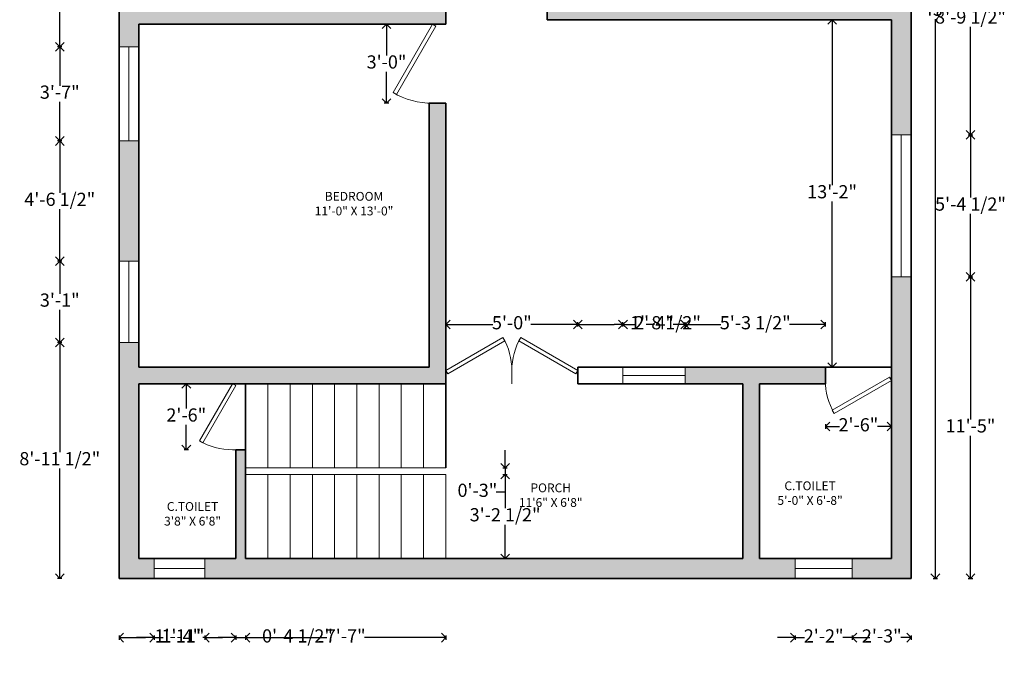
# Model space of a CAD drawing. Units: inches. Extents: x 2542 to 2989, y 529 to 1112.
# Tile 1 of 2: x 2542 to 2989, y 529 to 819. Entities that reach past the tile are written whole.
import ezdxf

# ---------------------------------------------------------------- set-up
doc = ezdxf.new("R2010")
doc.units = ezdxf.units.IN
for name, color, linetype, lineweight in [('A-ANNO-DIMS', 2, 'Continuous', 18), ('A-AREA-IDEN', 7, 'Continuous', 18), ('A-DOOR', 3, 'Continuous', 18), ('A-FLOR-STRS', 7, 'Continuous', 18), ('A-GLAZ', 4, 'Continuous', 18), ('A-WALL', 7, 'Continuous', 35)]:
    doc.layers.add(name, color=color, linetype=linetype, lineweight=lineweight)
doc.layers.add('A-WALL-PATT', color=30, linetype='Continuous', lineweight=13, true_color=0xf26722)
doc.styles.get("Standard").update_dxf_attribs({"font": 'arial.ttf'})
doc.dimstyles.new('ISO-25', dxfattribs={"dimtxt": 6, "dimasz": 4, "dimexe": 1, "dimexo": 1, "dimtad": 0, "dimtih": 1, "dimtoh": 1, "dimlunit": 3, "dimtxsty": 'Standard', "dimblk": 'OPEN90', "dimcen": 2.5, "dimadec": 0, "dimazin": 0, "dimtfac": 1, "dimtmove": 0, "dimatfit": 3, "dimfxl": 1, "dimfxlon": 1, "dimarcsym": 0})

# ---------------------------------------------------------------- blocks, each defined once
blk = doc.blocks.new('*U8')
for p, q in [((-30, 0), (-30, -6)), ((0, 0), (0, -6))]:
    blk.add_line(p, q)
blk.add_lwpolyline([(0, 0), (-25.98, 15), (-26.86, 13.48), (-0.88, -1.52)], close=True)
blk.add_arc((0, 0), 30, 150, 180)
blk = doc.blocks.new('*U9')
for p, q in [((0, 0), (0, -6)), ((30, 0), (30, -6))]:
    blk.add_line(p, q)
blk.add_lwpolyline([(0, 0), (25.98, 15), (26.86, 13.48), (0.87, -1.52)], close=True)
blk.add_arc((0, 0), 30, 0, 30)
blk = doc.blocks.new('*U6')
for p, q in [((-30, 0), (-30, 6)), ((0, 0), (0, 6))]:
    blk.add_line(p, q)
blk.add_lwpolyline([(0, 0), (-25.98, -15), (-26.86, -13.48), (-0.88, 1.52)], close=True)
blk.add_arc((0, 0), 30, 180, 210)
blk = doc.blocks.new('*U7')
for p, q in [((0, 0), (0, 6)), ((30, 0), (30, 6))]:
    blk.add_line(p, q)
blk.add_lwpolyline([(0, 0), (25.98, -15), (26.86, -13.48), (0.87, 1.52)], close=True)
blk.add_arc((0, 0), 30, 330, 0)
blk = doc.blocks.new('*U4')
for p, q in [((0, 0), (0, -6)), ((-36, 0), (-36, -6))]:
    blk.add_line(p, q)
blk.add_lwpolyline([(0, 0), (-31.18, 18), (-32.05, 16.48), (-0.88, -1.52)], close=True)
blk.add_arc((0, 0), 36, 150, 180)
blk = doc.blocks.new('_Open90')
at = {"color": 0, "linetype": 'ByBlock', "lineweight": -2}
for p, q in [((0, 0), (-1, 0)), ((-0.5, 0.5), (0, 0)), ((0, 0), (-0.5, -0.5))]:
    blk.add_line(p, q, dxfattribs=at)
blk = doc.blocks.new('*D13')
at = {"layer": 'A-ANNO-DIMS', "color": 0, "lineweight": -2, "transparency": 16777216}
for p, q in [((2957.03, 1081), (2959.03, 1081)), ((2958.03, 1077), (2958.03, 826.69)), ((2958.03, 569), (2958.03, 819.31)), ((2957.03, 565), (2959.03, 565))]:
    blk.add_line(p, q, dxfattribs=at)
at = {"layer": 'Defpoints', "color": 0, "transparency": 16777216}
for p in [(2947.06, 1081), (2947.06, 565), (2958.03, 565)]:
    blk.add_point(p, dxfattribs=at)
at = {"layer": 'A-ANNO-DIMS', "color": 0, "lineweight": -2, "transparency": 16777216, "xscale": 4, "yscale": 4, "zscale": 4}
for p, rotation in [((2958.03, 1081), 90), ((2958.03, 565), 270)]:
    blk.add_blockref('_Open90', p, dxfattribs=dict(at, rotation=rotation))
at = {"layer": 'A-ANNO-DIMS', "color": 0, "transparency": 16777216, "insert": (2958.03, 823), "char_height": 6, "attachment_point": 5}
blk.add_mtext("43'", dxfattribs=at)
blk = doc.blocks.new('*D14')
at = {"layer": 'A-ANNO-DIMS', "color": 0, "lineweight": -2, "transparency": 16777216}
for p, q in [((2561.11, 672.25), (2559.11, 672.25)), ((2560.11, 668.25), (2560.11, 622.35)), ((2560.11, 569), (2560.11, 614.9)), ((2561.11, 565), (2559.11, 565))]:
    blk.add_line(p, q, dxfattribs=at)
at = {"layer": 'Defpoints', "color": 0, "transparency": 16777216}
for p in [(2560.11, 672.25), (2587.06, 672.25), (2587.06, 565)]:
    blk.add_point(p, dxfattribs=at)
at = {"layer": 'A-ANNO-DIMS', "color": 0, "lineweight": -2, "transparency": 16777216, "xscale": 4, "yscale": 4, "zscale": 4}
for p, rotation in [((2560.11, 672.25), 90), ((2560.11, 565), 270)]:
    blk.add_blockref('_Open90', p, dxfattribs=dict(at, rotation=rotation))
at = {"layer": 'A-ANNO-DIMS', "color": 0, "transparency": 16777216, "insert": (2560.11, 618.63), "char_height": 6, "attachment_point": 5}
blk.add_mtext('8\'-11 1/2"', dxfattribs=at)
blk = doc.blocks.new('*D15')
at = {"layer": 'A-ANNO-DIMS', "color": 0, "lineweight": -2, "transparency": 16777216}
for p, q in [((2561.11, 709.22), (2559.11, 709.22)), ((2560.11, 705.22), (2560.11, 694.43)), ((2560.11, 676.25), (2560.11, 687.05)), ((2561.11, 672.25), (2559.11, 672.25))]:
    blk.add_line(p, q, dxfattribs=at)
at = {"layer": 'Defpoints', "color": 0, "transparency": 16777216}
for p in [(2560.11, 709.22), (2587.06, 709.22), (2587.06, 672.25)]:
    blk.add_point(p, dxfattribs=at)
at = {"layer": 'A-ANNO-DIMS', "color": 0, "lineweight": -2, "transparency": 16777216, "xscale": 4, "yscale": 4, "zscale": 4}
for p, rotation in [((2560.11, 709.22), 90), ((2560.11, 672.25), 270)]:
    blk.add_blockref('_Open90', p, dxfattribs=dict(at, rotation=rotation))
at = {"layer": 'A-ANNO-DIMS', "color": 0, "transparency": 16777216, "insert": (2560.11, 690.74), "char_height": 6, "attachment_point": 5}
blk.add_mtext('3\'-1"', dxfattribs=at)
blk = doc.blocks.new('*D16')
at = {"layer": 'A-ANNO-DIMS', "color": 0, "lineweight": -2, "transparency": 16777216}
for p, q in [((2561.11, 763.87), (2559.11, 763.87)), ((2560.11, 759.87), (2560.11, 740.27)), ((2560.11, 713.22), (2560.11, 732.82)), ((2561.11, 709.22), (2559.11, 709.22))]:
    blk.add_line(p, q, dxfattribs=at)
at = {"layer": 'Defpoints', "color": 0, "transparency": 16777216}
for p in [(2560.11, 763.87), (2587.06, 763.87), (2587.06, 709.22)]:
    blk.add_point(p, dxfattribs=at)
at = {"layer": 'A-ANNO-DIMS', "color": 0, "lineweight": -2, "transparency": 16777216, "xscale": 4, "yscale": 4, "zscale": 4}
for p, rotation in [((2560.11, 763.87), 90), ((2560.11, 709.22), 270)]:
    blk.add_blockref('_Open90', p, dxfattribs=dict(at, rotation=rotation))
at = {"layer": 'A-ANNO-DIMS', "color": 0, "transparency": 16777216, "insert": (2560.11, 736.55), "char_height": 6, "attachment_point": 5}
blk.add_mtext('4\'-6 1/2"', dxfattribs=at)
blk = doc.blocks.new('*D17')
at = {"layer": 'A-ANNO-DIMS', "color": 0, "lineweight": -2, "transparency": 16777216}
for p, q in [((2561.11, 806.69), (2559.11, 806.69)), ((2560.11, 802.69), (2560.11, 788.97)), ((2560.11, 767.87), (2560.11, 781.59)), ((2561.11, 763.87), (2559.11, 763.87))]:
    blk.add_line(p, q, dxfattribs=at)
at = {"layer": 'Defpoints', "color": 0, "transparency": 16777216}
for p in [(2560.11, 806.69), (2587.06, 806.69), (2587.06, 763.87)]:
    blk.add_point(p, dxfattribs=at)
at = {"layer": 'A-ANNO-DIMS', "color": 0, "lineweight": -2, "transparency": 16777216, "xscale": 4, "yscale": 4, "zscale": 4}
for p, rotation in [((2560.11, 806.69), 90), ((2560.11, 763.87), 270)]:
    blk.add_blockref('_Open90', p, dxfattribs=dict(at, rotation=rotation))
at = {"layer": 'A-ANNO-DIMS', "color": 0, "transparency": 16777216, "insert": (2560.11, 785.28), "char_height": 6, "attachment_point": 5}
blk.add_mtext('3\'-7"', dxfattribs=at)
blk = doc.blocks.new('*D18')
at = {"layer": 'A-ANNO-DIMS', "color": 0, "lineweight": -2, "transparency": 16777216}
for p, q in [((2561.11, 866.43), (2559.11, 866.43)), ((2560.11, 862.43), (2560.11, 840.29)), ((2560.11, 810.69), (2560.11, 832.83)), ((2561.11, 806.69), (2559.11, 806.69))]:
    blk.add_line(p, q, dxfattribs=at)
at = {"layer": 'Defpoints', "color": 0, "transparency": 16777216}
for p in [(2560.11, 866.43), (2587.06, 866.43), (2587.06, 806.69)]:
    blk.add_point(p, dxfattribs=at)
at = {"layer": 'A-ANNO-DIMS', "color": 0, "lineweight": -2, "transparency": 16777216, "xscale": 4, "yscale": 4, "zscale": 4}
for p, rotation in [((2560.11, 866.43), 90), ((2560.11, 806.69), 270)]:
    blk.add_blockref('_Open90', p, dxfattribs=dict(at, rotation=rotation))
at = {"layer": 'A-ANNO-DIMS', "color": 0, "transparency": 16777216, "insert": (2560.11, 836.56), "char_height": 6, "attachment_point": 5}
blk.add_mtext('4\'-11 1/2"', dxfattribs=at)
blk = doc.blocks.new('*D23')
at = {"layer": 'A-ANNO-DIMS', "color": 0, "lineweight": -2, "transparency": 16777216}
for p, q in [((2973.01, 702.1), (2975.01, 702.1)), ((2974.01, 698.1), (2974.01, 637.24)), ((2974.01, 569), (2974.01, 629.86)), ((2973.01, 565), (2975.01, 565))]:
    blk.add_line(p, q, dxfattribs=at)
at = {"layer": 'Defpoints', "color": 0, "transparency": 16777216}
for p in [(2947.06, 702.1), (2974.01, 702.1), (2947.06, 565)]:
    blk.add_point(p, dxfattribs=at)
at = {"layer": 'A-ANNO-DIMS', "color": 0, "lineweight": -2, "transparency": 16777216, "xscale": 4, "yscale": 4, "zscale": 4}
for p, rotation in [((2974.01, 702.1), 90), ((2974.01, 565), 270)]:
    blk.add_blockref('_Open90', p, dxfattribs=dict(at, rotation=rotation))
at = {"layer": 'A-ANNO-DIMS', "color": 0, "transparency": 16777216, "insert": (2974.01, 633.55), "char_height": 6, "attachment_point": 5}
blk.add_mtext('11\'-5"', dxfattribs=at)
blk = doc.blocks.new('*D24')
at = {"layer": 'A-ANNO-DIMS', "color": 0, "lineweight": -2, "transparency": 16777216}
for p, q in [((2973.01, 766.68), (2975.01, 766.68)), ((2974.01, 762.68), (2974.01, 738.11)), ((2974.01, 706.1), (2974.01, 730.66)), ((2973.01, 702.1), (2975.01, 702.1))]:
    blk.add_line(p, q, dxfattribs=at)
at = {"layer": 'Defpoints', "color": 0, "transparency": 16777216}
for p in [(2947.06, 766.68), (2974.01, 766.68), (2947.06, 702.1)]:
    blk.add_point(p, dxfattribs=at)
at = {"layer": 'A-ANNO-DIMS', "color": 0, "lineweight": -2, "transparency": 16777216, "xscale": 4, "yscale": 4, "zscale": 4}
for p, rotation in [((2974.01, 766.68), 90), ((2974.01, 702.1), 270)]:
    blk.add_blockref('_Open90', p, dxfattribs=dict(at, rotation=rotation))
at = {"layer": 'A-ANNO-DIMS', "color": 0, "transparency": 16777216, "insert": (2974.01, 734.39), "char_height": 6, "attachment_point": 5}
blk.add_mtext('5\'-4 1/2"', dxfattribs=at)
blk = doc.blocks.new('*D25')
at = {"layer": 'A-ANNO-DIMS', "color": 0, "lineweight": -2, "transparency": 16777216}
for p, q in [((2973.01, 872.19), (2975.01, 872.19)), ((2974.01, 868.19), (2974.01, 823.16)), ((2974.01, 770.68), (2974.01, 815.71)), ((2973.01, 766.68), (2975.01, 766.68))]:
    blk.add_line(p, q, dxfattribs=at)
at = {"layer": 'Defpoints', "color": 0, "transparency": 16777216}
for p in [(2947.06, 872.19), (2974.01, 872.19), (2947.06, 766.68)]:
    blk.add_point(p, dxfattribs=at)
at = {"layer": 'A-ANNO-DIMS', "color": 0, "lineweight": -2, "transparency": 16777216, "xscale": 4, "yscale": 4, "zscale": 4}
for p, rotation in [((2974.01, 872.19), 90), ((2974.01, 766.68), 270)]:
    blk.add_blockref('_Open90', p, dxfattribs=dict(at, rotation=rotation))
at = {"layer": 'A-ANNO-DIMS', "color": 0, "transparency": 16777216, "insert": (2974.01, 819.43), "char_height": 6, "attachment_point": 5}
blk.add_mtext('8\'-9 1/2"', dxfattribs=at)
blk = doc.blocks.new('*D30')
at = {"layer": 'A-ANNO-DIMS', "color": 0, "lineweight": -2, "transparency": 16777216}
for p, q in [((2587.06, 539.05), (2587.06, 537.05)), ((2591.06, 538.05), (2599.04, 538.05)), ((2603.04, 539.05), (2603.04, 537.05)), ((2603.04, 538.05), (2607.04, 538.05))]:
    blk.add_line(p, q, dxfattribs=at)
at = {"layer": 'Defpoints', "color": 0, "transparency": 16777216}
for p in [(2587.06, 565), (2603.04, 565), (2603.04, 538.05)]:
    blk.add_point(p, dxfattribs=at)
at = {"layer": 'A-ANNO-DIMS', "color": 0, "lineweight": -2, "transparency": 16777216, "xscale": 4, "yscale": 4, "zscale": 4, "rotation": 180}
blk.add_blockref('_Open90', (2587.06, 538.05), dxfattribs=at)
at = {"layer": 'A-ANNO-DIMS', "color": 0, "lineweight": -2, "transparency": 16777216, "xscale": 4, "yscale": 4, "zscale": 4}
blk.add_blockref('_Open90', (2603.04, 538.05), dxfattribs=at)
at = {"layer": 'A-ANNO-DIMS', "color": 0, "transparency": 16777216, "insert": (2615.36, 538.05), "char_height": 6, "attachment_point": 5}
blk.add_mtext('1\'-4"', dxfattribs=at)
blk = doc.blocks.new('*D31')
at = {"layer": 'A-ANNO-DIMS', "color": 0, "lineweight": -2, "transparency": 16777216}
for p, q in [((2599.04, 538.05), (2595.04, 538.05)), ((2603.04, 539.05), (2603.04, 537.05)), ((2603.04, 538.05), (2603.87, 538.05)), ((2626, 538.05), (2625.17, 538.05)), ((2626, 539.05), (2626, 537.05)), ((2630, 538.05), (2634, 538.05))]:
    blk.add_line(p, q, dxfattribs=at)
at = {"layer": 'Defpoints', "color": 0, "transparency": 16777216}
for p in [(2603.04, 565), (2626, 565), (2626, 538.05)]:
    blk.add_point(p, dxfattribs=at)
at = {"layer": 'A-ANNO-DIMS', "color": 0, "lineweight": -2, "transparency": 16777216, "xscale": 4, "yscale": 4, "zscale": 4}
blk.add_blockref('_Open90', (2603.04, 538.05), dxfattribs=at)
at = {"layer": 'A-ANNO-DIMS', "color": 0, "lineweight": -2, "transparency": 16777216, "xscale": 4, "yscale": 4, "zscale": 4, "rotation": 180}
blk.add_blockref('_Open90', (2626, 538.05), dxfattribs=at)
at = {"layer": 'A-ANNO-DIMS', "color": 0, "transparency": 16777216, "insert": (2614.52, 538.05), "char_height": 6, "attachment_point": 5}
blk.add_mtext('1\'-11"', dxfattribs=at)
blk = doc.blocks.new('*D32')
at = {"layer": 'A-ANNO-DIMS', "color": 0, "lineweight": -2, "transparency": 16777216}
for p, q in [((2890.27, 538.05), (2886.27, 538.05)), ((2894.27, 539.05), (2894.27, 537.05)), ((2894.27, 538.05), (2898.63, 538.05)), ((2920.3, 538.05), (2915.93, 538.05)), ((2920.3, 539.05), (2920.3, 537.05)), ((2924.3, 538.05), (2928.3, 538.05))]:
    blk.add_line(p, q, dxfattribs=at)
at = {"layer": 'Defpoints', "color": 0, "transparency": 16777216}
for p in [(2894.27, 565), (2920.3, 565), (2920.3, 538.05)]:
    blk.add_point(p, dxfattribs=at)
at = {"layer": 'A-ANNO-DIMS', "color": 0, "lineweight": -2, "transparency": 16777216, "xscale": 4, "yscale": 4, "zscale": 4}
blk.add_blockref('_Open90', (2894.27, 538.05), dxfattribs=at)
at = {"layer": 'A-ANNO-DIMS', "color": 0, "lineweight": -2, "transparency": 16777216, "xscale": 4, "yscale": 4, "zscale": 4, "rotation": 180}
blk.add_blockref('_Open90', (2920.3, 538.05), dxfattribs=at)
at = {"layer": 'A-ANNO-DIMS', "color": 0, "transparency": 16777216, "insert": (2907.28, 538.05), "char_height": 6, "attachment_point": 5}
blk.add_mtext('2\'-2"', dxfattribs=at)
blk = doc.blocks.new('*D33')
at = {"layer": 'A-ANNO-DIMS', "color": 0, "lineweight": -2, "transparency": 16777216}
for p, q in [((2920.3, 539.05), (2920.3, 537.05)), ((2924.3, 538.05), (2925.03, 538.05)), ((2943.06, 538.05), (2942.33, 538.05)), ((2947.06, 539.05), (2947.06, 537.05))]:
    blk.add_line(p, q, dxfattribs=at)
at = {"layer": 'Defpoints', "color": 0, "transparency": 16777216}
for p in [(2920.3, 565), (2947.06, 565), (2947.06, 538.05)]:
    blk.add_point(p, dxfattribs=at)
at = {"layer": 'A-ANNO-DIMS', "color": 0, "lineweight": -2, "transparency": 16777216, "xscale": 4, "yscale": 4, "zscale": 4, "rotation": 180}
blk.add_blockref('_Open90', (2920.3, 538.05), dxfattribs=at)
at = {"layer": 'A-ANNO-DIMS', "color": 0, "lineweight": -2, "transparency": 16777216, "xscale": 4, "yscale": 4, "zscale": 4}
blk.add_blockref('_Open90', (2947.06, 538.05), dxfattribs=at)
at = {"layer": 'A-ANNO-DIMS', "color": 0, "transparency": 16777216, "insert": (2933.68, 538.05), "char_height": 6, "attachment_point": 5}
blk.add_mtext('2\'-3"', dxfattribs=at)
blk = doc.blocks.new('*D34')
at = {"layer": 'A-ANNO-DIMS', "color": 0, "lineweight": -2, "transparency": 16777216}
for p, q in [((2644.56, 539.05), (2644.56, 537.05)), ((2648.56, 538.05), (2681.48, 538.05)), ((2731.56, 538.05), (2698.63, 538.05)), ((2735.56, 539.05), (2735.56, 537.05))]:
    blk.add_line(p, q, dxfattribs=at)
at = {"layer": 'Defpoints', "color": 0, "transparency": 16777216}
for p in [(2644.56, 574), (2735.56, 574), (2735.56, 538.05)]:
    blk.add_point(p, dxfattribs=at)
at = {"layer": 'A-ANNO-DIMS', "color": 0, "lineweight": -2, "transparency": 16777216, "xscale": 4, "yscale": 4, "zscale": 4, "rotation": 180}
blk.add_blockref('_Open90', (2644.56, 538.05), dxfattribs=at)
at = {"layer": 'A-ANNO-DIMS', "color": 0, "lineweight": -2, "transparency": 16777216, "xscale": 4, "yscale": 4, "zscale": 4}
blk.add_blockref('_Open90', (2735.56, 538.05), dxfattribs=at)
at = {"layer": 'A-ANNO-DIMS', "color": 0, "transparency": 16777216, "insert": (2690.06, 538.05), "char_height": 6, "attachment_point": 5}
blk.add_mtext('7\'-7"', dxfattribs=at)
blk = doc.blocks.new('*D35')
at = {"layer": 'A-ANNO-DIMS', "color": 0, "lineweight": -2, "transparency": 16777216}
for p, q in [((2735.56, 679.45), (2735.56, 681.45)), ((2739.56, 680.45), (2756.96, 680.45)), ((2791.56, 680.45), (2774.16, 680.45)), ((2795.56, 679.45), (2795.56, 681.45))]:
    blk.add_line(p, q, dxfattribs=at)
at = {"layer": 'Defpoints', "color": 0, "transparency": 16777216}
for p in [(2795.56, 680.45), (2735.56, 653.5), (2795.56, 653.5)]:
    blk.add_point(p, dxfattribs=at)
at = {"layer": 'A-ANNO-DIMS', "color": 0, "lineweight": -2, "transparency": 16777216, "xscale": 4, "yscale": 4, "zscale": 4, "rotation": 180}
blk.add_blockref('_Open90', (2735.56, 680.45), dxfattribs=at)
at = {"layer": 'A-ANNO-DIMS', "color": 0, "lineweight": -2, "transparency": 16777216, "xscale": 4, "yscale": 4, "zscale": 4}
blk.add_blockref('_Open90', (2795.56, 680.45), dxfattribs=at)
at = {"layer": 'A-ANNO-DIMS', "color": 0, "transparency": 16777216, "insert": (2765.56, 680.45), "char_height": 6, "attachment_point": 5}
blk.add_mtext('5\'-0"', dxfattribs=at)
blk = doc.blocks.new('*D37')
at = {"layer": 'A-ANNO-DIMS', "color": 0, "lineweight": -2, "transparency": 16777216}
for p, q in [((2583.06, 833.64), (2579.06, 833.64)), ((2587.06, 832.64), (2587.06, 834.64)), ((2587.06, 833.64), (2596.06, 833.64)), ((2596.06, 832.64), (2596.06, 834.64)), ((2600.06, 833.64), (2604.06, 833.64))]:
    blk.add_line(p, q, dxfattribs=at)
at = {"layer": 'Defpoints', "color": 0, "transparency": 16777216}
for p in [(2596.06, 833.64), (2587.06, 806.69), (2596.06, 806.69)]:
    blk.add_point(p, dxfattribs=at)
at = {"layer": 'A-ANNO-DIMS', "color": 0, "lineweight": -2, "transparency": 16777216, "xscale": 4, "yscale": 4, "zscale": 4}
blk.add_blockref('_Open90', (2587.06, 833.64), dxfattribs=at)
at = {"layer": 'A-ANNO-DIMS', "color": 0, "lineweight": -2, "transparency": 16777216, "xscale": 4, "yscale": 4, "zscale": 4, "rotation": 180}
blk.add_blockref('_Open90', (2596.06, 833.64), dxfattribs=at)
at = {"layer": 'A-ANNO-DIMS', "color": 0, "transparency": 16777216, "insert": (2612.66, 833.64), "char_height": 6, "attachment_point": 5}
blk.add_mtext('0\'-9"', dxfattribs=at)
blk = doc.blocks.new('*D39')
at = {"layer": 'A-ANNO-DIMS', "color": 0, "lineweight": -2, "transparency": 16777216}
for p, q in [((2636.06, 538.05), (2632.06, 538.05)), ((2640.06, 539.05), (2640.06, 537.05)), ((2640.06, 538.05), (2644.56, 538.05)), ((2644.56, 539.05), (2644.56, 537.05)), ((2648.56, 538.05), (2652.56, 538.05))]:
    blk.add_line(p, q, dxfattribs=at)
at = {"layer": 'Defpoints', "color": 0, "transparency": 16777216}
for p in [(2640.06, 574), (2644.56, 574), (2644.56, 538.05)]:
    blk.add_point(p, dxfattribs=at)
at = {"layer": 'A-ANNO-DIMS', "color": 0, "lineweight": -2, "transparency": 16777216, "xscale": 4, "yscale": 4, "zscale": 4}
blk.add_blockref('_Open90', (2640.06, 538.05), dxfattribs=at)
at = {"layer": 'A-ANNO-DIMS', "color": 0, "lineweight": -2, "transparency": 16777216, "xscale": 4, "yscale": 4, "zscale": 4, "rotation": 180}
blk.add_blockref('_Open90', (2644.56, 538.05), dxfattribs=at)
at = {"layer": 'A-ANNO-DIMS', "color": 0, "transparency": 16777216, "insert": (2668.15, 538.05), "char_height": 6, "attachment_point": 5}
blk.add_mtext('0\'-4 1/2"', dxfattribs=at)
blk = doc.blocks.new('*D43')
at = {"layer": 'A-ANNO-DIMS', "color": 0, "lineweight": -2, "transparency": 16777216}
for p, q in [((2908.06, 635.05), (2908.06, 633.05)), ((2912.06, 634.05), (2914.41, 634.05)), ((2934.06, 634.05), (2931.71, 634.05)), ((2938.06, 635.05), (2938.06, 633.05))]:
    blk.add_line(p, q, dxfattribs=at)
at = {"layer": 'Defpoints', "color": 0, "transparency": 16777216}
for p in [(2908.06, 661), (2938.06, 661), (2908.06, 634.05)]:
    blk.add_point(p, dxfattribs=at)
at = {"layer": 'A-ANNO-DIMS', "color": 0, "lineweight": -2, "transparency": 16777216, "xscale": 4, "yscale": 4, "zscale": 4, "rotation": 180}
blk.add_blockref('_Open90', (2908.06, 634.05), dxfattribs=at)
at = {"layer": 'A-ANNO-DIMS', "color": 0, "lineweight": -2, "transparency": 16777216, "xscale": 4, "yscale": 4, "zscale": 4}
blk.add_blockref('_Open90', (2938.06, 634.05), dxfattribs=at)
at = {"layer": 'A-ANNO-DIMS', "color": 0, "transparency": 16777216, "insert": (2923.06, 634.05), "char_height": 6, "attachment_point": 5}
blk.add_mtext('2\'-6"', dxfattribs=at)
blk = doc.blocks.new('*D44')
at = {"layer": 'A-ANNO-DIMS', "color": 0, "lineweight": -2, "transparency": 16777216}
for p, q in [((2618.61, 653.5), (2616.61, 653.5)), ((2617.61, 649.5), (2617.61, 642.19)), ((2617.61, 627.5), (2617.61, 634.81)), ((2618.61, 623.5), (2616.61, 623.5))]:
    blk.add_line(p, q, dxfattribs=at)
at = {"layer": 'Defpoints', "color": 0, "transparency": 16777216}
for p in [(2617.61, 653.5), (2644.56, 653.5), (2644.56, 623.5)]:
    blk.add_point(p, dxfattribs=at)
at = {"layer": 'A-ANNO-DIMS', "color": 0, "lineweight": -2, "transparency": 16777216, "xscale": 4, "yscale": 4, "zscale": 4}
for p, rotation in [((2617.61, 653.5), 90), ((2617.61, 623.5), 270)]:
    blk.add_blockref('_Open90', p, dxfattribs=dict(at, rotation=rotation))
at = {"layer": 'A-ANNO-DIMS', "color": 0, "transparency": 16777216, "insert": (2617.61, 638.5), "char_height": 6, "attachment_point": 5}
blk.add_mtext('2\'-6"', dxfattribs=at)
blk = doc.blocks.new('*D45')
at = {"layer": 'A-ANNO-DIMS', "color": 0, "lineweight": -2, "transparency": 16777216}
for p, q in [((2816.07, 679.45), (2816.07, 681.45)), ((2820.07, 680.45), (2821.54, 680.45)), ((2840.32, 680.45), (2838.84, 680.45)), ((2844.32, 679.45), (2844.32, 681.45))]:
    blk.add_line(p, q, dxfattribs=at)
at = {"layer": 'Defpoints', "color": 0, "transparency": 16777216}
for p in [(2844.32, 680.45), (2816.07, 653.5), (2844.32, 653.5)]:
    blk.add_point(p, dxfattribs=at)
at = {"layer": 'A-ANNO-DIMS', "color": 0, "lineweight": -2, "transparency": 16777216, "xscale": 4, "yscale": 4, "zscale": 4, "rotation": 180}
blk.add_blockref('_Open90', (2816.07, 680.45), dxfattribs=at)
at = {"layer": 'A-ANNO-DIMS', "color": 0, "lineweight": -2, "transparency": 16777216, "xscale": 4, "yscale": 4, "zscale": 4}
blk.add_blockref('_Open90', (2844.32, 680.45), dxfattribs=at)
at = {"layer": 'A-ANNO-DIMS', "color": 0, "transparency": 16777216, "insert": (2830.19, 680.45), "char_height": 6, "attachment_point": 5}
blk.add_mtext('2\'-4"', dxfattribs=at)
blk = doc.blocks.new('*D46')
at = {"layer": 'A-ANNO-DIMS', "color": 0, "lineweight": -2, "transparency": 16777216}
for p, q in [((2795.56, 679.45), (2795.56, 681.45)), ((2799.56, 680.45), (2812.07, 680.45)), ((2816.07, 679.45), (2816.07, 681.45)), ((2816.07, 680.45), (2820.07, 680.45))]:
    blk.add_line(p, q, dxfattribs=at)
at = {"layer": 'Defpoints', "color": 0, "transparency": 16777216}
for p in [(2816.07, 680.45), (2795.56, 653.5), (2816.07, 653.5)]:
    blk.add_point(p, dxfattribs=at)
at = {"layer": 'A-ANNO-DIMS', "color": 0, "lineweight": -2, "transparency": 16777216, "xscale": 4, "yscale": 4, "zscale": 4, "rotation": 180}
blk.add_blockref('_Open90', (2795.56, 680.45), dxfattribs=at)
at = {"layer": 'A-ANNO-DIMS', "color": 0, "lineweight": -2, "transparency": 16777216, "xscale": 4, "yscale": 4, "zscale": 4}
blk.add_blockref('_Open90', (2816.07, 680.45), dxfattribs=at)
at = {"layer": 'A-ANNO-DIMS', "color": 0, "transparency": 16777216, "insert": (2835.38, 680.45), "char_height": 6, "attachment_point": 5}
blk.add_mtext('1\'-8 1/2"', dxfattribs=at)
blk = doc.blocks.new('*D47')
at = {"layer": 'A-ANNO-DIMS', "color": 0, "lineweight": -2, "transparency": 16777216}
for p, q in [((2844.32, 679.45), (2844.32, 681.45)), ((2848.32, 680.45), (2860.6, 680.45)), ((2904.06, 680.45), (2891.78, 680.45)), ((2908.06, 679.45), (2908.06, 681.45))]:
    blk.add_line(p, q, dxfattribs=at)
at = {"layer": 'Defpoints', "color": 0, "transparency": 16777216}
for p in [(2908.06, 680.45), (2844.32, 653.5), (2908.06, 653.5)]:
    blk.add_point(p, dxfattribs=at)
at = {"layer": 'A-ANNO-DIMS', "color": 0, "lineweight": -2, "transparency": 16777216, "xscale": 4, "yscale": 4, "zscale": 4, "rotation": 180}
blk.add_blockref('_Open90', (2844.32, 680.45), dxfattribs=at)
at = {"layer": 'A-ANNO-DIMS', "color": 0, "lineweight": -2, "transparency": 16777216, "xscale": 4, "yscale": 4, "zscale": 4}
blk.add_blockref('_Open90', (2908.06, 680.45), dxfattribs=at)
at = {"layer": 'A-ANNO-DIMS', "color": 0, "transparency": 16777216, "insert": (2876.19, 680.45), "char_height": 6, "attachment_point": 5}
blk.add_mtext('5\'-3 1/2"', dxfattribs=at)
blk = doc.blocks.new('*D48')
at = {"layer": 'A-ANNO-DIMS', "color": 0, "lineweight": -2, "transparency": 16777216}
for p, q in [((2709.61, 817), (2707.61, 817)), ((2708.61, 813), (2708.61, 802.69)), ((2708.61, 785), (2708.61, 795.31)), ((2709.61, 781), (2707.61, 781))]:
    blk.add_line(p, q, dxfattribs=at)
at = {"layer": 'Defpoints', "color": 0, "transparency": 16777216}
for p in [(2708.61, 817), (2735.56, 817), (2735.56, 781)]:
    blk.add_point(p, dxfattribs=at)
at = {"layer": 'A-ANNO-DIMS', "color": 0, "lineweight": -2, "transparency": 16777216, "xscale": 4, "yscale": 4, "zscale": 4}
for p, rotation in [((2708.61, 817), 90), ((2708.61, 781), 270)]:
    blk.add_blockref('_Open90', p, dxfattribs=dict(at, rotation=rotation))
at = {"layer": 'A-ANNO-DIMS', "color": 0, "transparency": 16777216, "insert": (2708.61, 799), "char_height": 6, "attachment_point": 5}
blk.add_mtext('3\'-0"', dxfattribs=at)
blk = doc.blocks.new('*D51')
at = {"layer": 'A-ANNO-DIMS', "color": 0, "lineweight": -2, "transparency": 16777216}
for p, q in [((2761.51, 612.25), (2763.51, 612.25)), ((2762.51, 608.25), (2762.51, 596.86)), ((2762.51, 578), (2762.51, 589.4)), ((2761.51, 574), (2763.51, 574))]:
    blk.add_line(p, q, dxfattribs=at)
at = {"layer": 'Defpoints', "color": 0, "transparency": 16777216}
for p in [(2735.56, 612.25), (2735.56, 574), (2762.51, 574)]:
    blk.add_point(p, dxfattribs=at)
at = {"layer": 'A-ANNO-DIMS', "color": 0, "lineweight": -2, "transparency": 16777216, "xscale": 4, "yscale": 4, "zscale": 4}
for p, rotation in [((2762.51, 612.25), 90), ((2762.51, 574), 270)]:
    blk.add_blockref('_Open90', p, dxfattribs=dict(at, rotation=rotation))
at = {"layer": 'A-ANNO-DIMS', "color": 0, "transparency": 16777216, "insert": (2762.51, 593.13), "char_height": 6, "attachment_point": 5}
blk.add_mtext('3\'-2 1/2"', dxfattribs=at)
blk = doc.blocks.new('*D52')
at = {"layer": 'A-ANNO-DIMS', "color": 0, "lineweight": -2, "transparency": 16777216}
for p, q in [((2762.51, 619.25), (2762.51, 623.25)), ((2761.51, 615.25), (2763.51, 615.25)), ((2762.51, 615.25), (2762.51, 612.25)), ((2761.51, 612.25), (2763.51, 612.25)), ((2762.51, 604.25), (2758.51, 604.25)), ((2762.51, 608.25), (2762.51, 604.25))]:
    blk.add_line(p, q, dxfattribs=at)
at = {"layer": 'Defpoints', "color": 0, "transparency": 16777216}
for p in [(2735.56, 615.25), (2735.56, 612.25), (2762.51, 612.25)]:
    blk.add_point(p, dxfattribs=at)
at = {"layer": 'A-ANNO-DIMS', "color": 0, "lineweight": -2, "transparency": 16777216, "xscale": 4, "yscale": 4, "zscale": 4}
for p, rotation in [((2762.51, 615.25), 270), ((2762.51, 612.25), 90)]:
    blk.add_blockref('_Open90', p, dxfattribs=dict(at, rotation=rotation))
at = {"layer": 'A-ANNO-DIMS', "color": 0, "transparency": 16777216, "insert": (2749.91, 604.25), "char_height": 6, "attachment_point": 5}
blk.add_mtext('0\'-3"', dxfattribs=at)
blk = doc.blocks.new('*D53')
at = {"layer": 'A-ANNO-DIMS', "color": 0, "lineweight": -2, "transparency": 16777216}
for p, q in [((2912.11, 819), (2910.11, 819)), ((2911.11, 815), (2911.11, 743.69)), ((2911.11, 665), (2911.11, 736.31)), ((2912.11, 661), (2910.11, 661))]:
    blk.add_line(p, q, dxfattribs=at)
at = {"layer": 'Defpoints', "color": 0, "transparency": 16777216}
for p in [(2911.11, 819), (2938.06, 819), (2938.06, 661)]:
    blk.add_point(p, dxfattribs=at)
at = {"layer": 'A-ANNO-DIMS', "color": 0, "lineweight": -2, "transparency": 16777216, "xscale": 4, "yscale": 4, "zscale": 4}
for p, rotation in [((2911.11, 819), 90), ((2911.11, 661), 270)]:
    blk.add_blockref('_Open90', p, dxfattribs=dict(at, rotation=rotation))
at = {"layer": 'A-ANNO-DIMS', "color": 0, "transparency": 16777216, "insert": (2911.11, 740), "char_height": 6, "attachment_point": 5}
blk.add_mtext('13\'-2"', dxfattribs=at)

msp = doc.modelspace()

# ---------------------------------------------------------------- hatches: boundary and pattern name
at = {"layer": 'A-WALL-PATT'}
h = msp.add_hatch(color=256, dxfattribs=at)
h.dxf.hatch_style = 1
h.paths.add_polyline_path([(2947.06, 1081.002), (2587.06, 1081.002), (2587.06, 1040.94), (2596.06, 1040.94), (2596.06, 1072.002), (2726.06, 1072.002), (2726.06, 1027.002), (2726.093, 1027.002), (2733.56, 1027.002), (2733.56, 1072.002), (2836.56, 1072.002), (2836.56, 997.002), (2732.067, 997.002), (2732.06, 996.988), (2726.06, 997.002), (2726.06, 989.502), (2781.56, 989.502), (2781.56, 862.502), (2787.56, 862.502), (2789.06, 862.502), (2789.06, 989.502), (2844.06, 989.502), (2844.06, 995.502), (2844.06, 1072.002), (2938.06, 1072.002), (2938.06, 1057.232), (2947.06, 1057.232)])
h.paths.add_polyline_path([(2596.06, 944.502), (2728.06, 944.502), (2728.06, 860.502), (2735.56, 860.502), (2735.56, 952.002), (2729.56, 952.002), (2596.06, 952.002), (2596.06, 986.938), (2587.06, 986.938), (2587.06, 920.709), (2596.06, 920.709)])
h.paths.add_polyline_path([(2735.56, 824.502), (2729.56, 824.502), (2596.06, 824.502), (2596.06, 866.432), (2587.06, 866.432), (2587.06, 806.686), (2596.06, 806.686), (2596.06, 817.002), (2735.56, 817.002)])
h.paths.add_polyline_path([(2596.06, 763.869), (2587.06, 763.869), (2587.06, 709.221), (2596.06, 709.221)], flags=17)
h.paths.add_polyline_path([(2596.06, 653.502), (2735.56, 653.502), (2735.56, 659.502), (2735.56, 781.002), (2729.56, 781.002), (2728.06, 781.002), (2728.06, 661.002), (2596.06, 661.002), (2596.06, 672.254), (2587.06, 672.254), (2587.06, 565.002), (2603.045, 565.002), (2603.045, 574.002), (2596.06, 574.002)])
h.paths.add_polyline_path([(2894.269, 574.002), (2878.06, 574.002), (2878.06, 653.502), (2908.06, 653.502), (2908.06, 661.002), (2844.316, 661.002), (2844.316, 653.502), (2870.56, 653.502), (2870.56, 574.002), (2644.56, 574.002), (2644.56, 623.502), (2640.06, 623.502), (2640.06, 574.002), (2625.996, 574.002), (2625.996, 565.002), (2894.269, 565.002)])
h.paths.add_polyline_path([(2947.06, 702.099), (2938.06, 702.099), (2938.06, 574.002), (2920.298, 574.002), (2920.298, 565.002), (2947.06, 565.002)])
h.paths.add_polyline_path([(2947.06, 1021.275), (2938.06, 1021.275), (2938.06, 997.002), (2876.06, 997.002), (2876.06, 989.502), (2938.06, 989.502), (2938.06, 945.972), (2947.06, 945.972)], flags=17)
h.paths.add_polyline_path([(2947.06, 872.193), (2938.06, 872.193), (2938.06, 826.502), (2781.56, 826.502), (2781.56, 819.002), (2938.06, 819.002), (2938.06, 766.676), (2947.06, 766.676)])

# ---------------------------------------------------------------- linework, layer by layer
at = {"layer": 'A-FLOR-STRS'}
for p, q in [((2654.671, 653.502), (2654.671, 615.252)), ((2664.782, 653.502), (2664.782, 615.252)), ((2674.893, 653.502), (2674.893, 615.252)), ((2685.004, 653.502), (2685.004, 615.252)), ((2695.115, 653.502), (2695.115, 615.252)), ((2705.226, 653.502), (2705.226, 615.252)), ((2715.337, 653.502), (2715.337, 615.252)), ((2725.449, 653.502), (2725.449, 615.252)), ((2735.56, 615.252), (2644.56, 615.252)), ((2735.56, 612.252), (2644.56, 612.252)), ((2654.671, 612.252), (2654.671, 574.002)), ((2664.782, 612.252), (2664.782, 574.002)), ((2674.893, 612.252), (2674.893, 574.002)), ((2685.004, 612.252), (2685.004, 574.002)), ((2695.115, 612.252), (2695.115, 574.002)), ((2705.226, 612.252), (2705.226, 574.002)), ((2715.337, 612.252), (2715.337, 574.002)), ((2725.449, 612.252), (2725.449, 574.002)), ((2735.56, 612.252), (2735.56, 574.002))]:
    msp.add_line(p, q, dxfattribs=at)
at = {"layer": 'A-GLAZ'}
for p, q in [((2596.06, 806.686), (2587.06, 806.686)), ((2591.56, 763.869), (2591.56, 806.686)), ((2938.06, 766.676), (2947.06, 766.676)), ((2942.56, 702.099), (2942.56, 766.676)), ((2596.06, 763.869), (2587.06, 763.869)), ((2587.06, 709.221), (2596.06, 709.221)), ((2591.56, 709.221), (2591.56, 672.254)), ((2938.06, 702.099), (2947.06, 702.099)), ((2596.06, 672.254), (2587.06, 672.254)), ((2816.069, 661.002), (2816.069, 653.502)), ((2844.316, 661.002), (2844.316, 653.502)), ((2844.316, 657.252), (2816.069, 657.252)), ((2603.045, 574.002), (2603.045, 565.002)), ((2625.996, 574.002), (2625.996, 565.002)), ((2894.269, 574.002), (2894.269, 565.002)), ((2920.298, 574.002), (2920.298, 565.002)), ((2625.996, 569.502), (2603.045, 569.502)), ((2920.298, 569.502), (2894.269, 569.502))]:
    msp.add_line(p, q, dxfattribs=at)
at = {"layer": 'A-WALL'}
for p, q in [((2587.06, 1081.002), (2587.06, 565.002)), ((2947.06, 565.002), (2947.06, 1081.002)), ((2735.56, 824.502), (2735.56, 817.002)), ((2781.56, 826.502), (2781.56, 819.002)), ((2938.06, 819.002), (2781.56, 819.002)), ((2938.06, 574.002), (2938.06, 819.002)), ((2596.06, 817.002), (2735.56, 817.002)), ((2596.06, 817.002), (2596.06, 661.002)), ((2728.06, 781.002), (2728.06, 661.002)), ((2728.06, 781.002), (2735.56, 781.002)), ((2735.56, 781.002), (2735.56, 615.252)), ((2596.06, 661.002), (2728.06, 661.002)), ((2795.56, 661.002), (2938.06, 661.002)), ((2795.56, 661.002), (2795.56, 653.502)), ((2908.06, 653.502), (2908.06, 661.002)), ((2596.06, 653.502), (2735.56, 653.502)), ((2596.06, 653.502), (2596.06, 574.002)), ((2644.56, 653.502), (2644.56, 574.002)), ((2795.56, 653.502), (2870.56, 653.502)), ((2870.56, 574.002), (2870.56, 653.502)), ((2878.06, 574.002), (2878.06, 653.502)), ((2878.06, 653.502), (2908.06, 653.502)), ((2640.06, 623.502), (2640.06, 574.002)), ((2644.56, 623.502), (2640.06, 623.502)), ((2596.06, 574.002), (2640.06, 574.002)), ((2644.56, 574.002), (2870.56, 574.002)), ((2878.06, 574.002), (2938.06, 574.002)), ((2587.06, 565.002), (2947.06, 565.002))]:
    msp.add_line(p, q, dxfattribs=at)

# ---------------------------------------------------------------- block references
at = {"layer": 'A-DOOR'}
for name, p, rotation in [('*U4', (2729.56, 817.002), 90), ('*U7', (2638.56, 653.502), 270)]:
    msp.add_blockref(name, p, dxfattribs=dict(at, rotation=rotation))
for name, p in [('*U9', (2735.56, 659.502)), ('*U8', (2795.56, 659.502)), ('*U6', (2938.06, 655.002))]:
    msp.add_blockref(name, p, dxfattribs=at)

# ---------------------------------------------------------------- texts
at = {"layer": 'A-AREA-IDEN', "char_height": 4, "attachment_point": 1}
for s, insert in [('\\pxqc;BEDROOM\\P11\'-0" X 13\'-0"', (2659.637, 740.69)), ('\\pxqc;C.TOILET\\P5\'-0" X 6\'-8"', (2866.893, 609.088)), ('\\pxqc;PORCH\\P11\'6" X 6\'8"', (2749.025, 608.161)), ('\\pxqc;C.TOILET\\P3\'8" X 6\'8"', (2586.248, 599.685))]:
    msp.add_mtext_dynamic_manual_height_columns(s, width=68.42278, gutter_width=12.5, heights=[0], dxfattribs=dict(at, insert=insert))

# ---------------------------------------------------------------- dimensions: what is measured, and where the dimension line sits
at = {"layer": 'A-ANNO-DIMS'}
for base, p1, p2, angle, override, picture, middle in [((2958.029, 565.002), (2947.06, 1081.002), (2947.06, 565.002), 90, {"dimclrd": 0, "dimclre": 0, "dimclrt": 0}, '*D13', (2958.029, 823.002)), ((2974.01, 872.193), (2947.06, 766.676), (2947.06, 872.193), 90, {"dimdec": 1, "dimlfac": 1, "dimrnd": 0, "dimzin": 1, "dimdsep": 46, "dimlunit": 4, "dimfrac": 2}, '*D25', (2974.01, 819.435)), ((2560.11, 866.432), (2587.06, 806.686), (2587.06, 866.432), 90, {"dimdec": 1, "dimlfac": 1, "dimrnd": 0, "dimzin": 1, "dimdsep": 46, "dimlunit": 4, "dimfrac": 2}, '*D18', (2560.11, 836.559)), ((2911.11, 819.002), (2938.06, 661.002), (2938.06, 819.002), 90, {"dimdec": 1, "dimlfac": 1, "dimrnd": 0, "dimzin": 1, "dimdsep": 46, "dimlunit": 4, "dimfrac": 2}, '*D53', (2911.11, 740.002)), ((2708.61, 817.002), (2735.56, 781.002), (2735.56, 817.002), 90, {"dimdec": 1, "dimlfac": 1, "dimrnd": 0, "dimzin": 1, "dimdsep": 46, "dimlunit": 4, "dimfrac": 2}, '*D48', (2708.61, 799.002)), ((2560.11, 806.686), (2587.06, 763.869), (2587.06, 806.686), 90, {"dimdec": 1, "dimlfac": 1, "dimrnd": 0, "dimzin": 1, "dimdsep": 46, "dimlunit": 4, "dimfrac": 2}, '*D17', (2560.11, 785.278)), ((2974.01, 766.676), (2947.06, 702.099), (2947.06, 766.676), 90, {"dimdec": 1, "dimlfac": 1, "dimrnd": 0, "dimzin": 1, "dimdsep": 46, "dimlunit": 4, "dimfrac": 2}, '*D24', (2974.01, 734.388)), ((2560.11, 763.869), (2587.06, 709.221), (2587.06, 763.869), 90, {"dimdec": 1, "dimlfac": 1, "dimrnd": 0, "dimzin": 1, "dimdsep": 46, "dimlunit": 4, "dimfrac": 2}, '*D16', (2560.11, 736.545)), ((2560.11, 709.221), (2587.06, 672.254), (2587.06, 709.221), 90, {"dimdec": 1, "dimlfac": 1, "dimrnd": 0, "dimzin": 1, "dimdsep": 46, "dimlunit": 4, "dimfrac": 2}, '*D15', (2560.11, 690.738)), ((2974.01, 702.099), (2947.06, 565.002), (2947.06, 702.099), 90, {"dimdec": 1, "dimlfac": 1, "dimrnd": 0, "dimzin": 1, "dimdsep": 46, "dimlunit": 4, "dimfrac": 2}, '*D23', (2974.01, 633.55)), ((2560.11, 672.254), (2587.06, 565.002), (2587.06, 672.254), 90, {"dimdec": 1, "dimlfac": 1, "dimrnd": 0, "dimzin": 1, "dimdsep": 46, "dimlunit": 4, "dimfrac": 2}, '*D14', (2560.11, 618.628)), ((2908.06, 634.052), (2938.06, 661.002), (2908.06, 661.002), 180, {"dimdec": 1, "dimlfac": 1, "dimrnd": 0, "dimzin": 1, "dimdsep": 46, "dimlunit": 4, "dimfrac": 2}, '*D43', (2923.06, 634.052)), ((2617.61, 653.502), (2644.56, 623.502), (2644.56, 653.502), 90, {"dimdec": 1, "dimlfac": 1, "dimrnd": 0, "dimzin": 1, "dimdsep": 46, "dimlunit": 4, "dimfrac": 2}, '*D44', (2617.61, 638.502)), ((2762.51, 612.252), (2735.56, 615.252), (2735.56, 612.252), 270, {"dimdec": 1, "dimlfac": 1, "dimrnd": 0, "dimzin": 1, "dimdsep": 46, "dimlunit": 4, "dimfrac": 2}, '*D52', (2749.91, 604.252)), ((2762.509656, 574.001653), (2735.559656, 612.251653), (2735.559656, 574.001653), 270, {"dimdec": 1, "dimlfac": 1, "dimrnd": 0, "dimzin": 1, "dimdsep": 46, "dimlunit": 4, "dimfrac": 2}, '*D51', (2762.509656, 593.126653))]:
    dim = msp.add_linear_dim(base=base, p1=p1, p2=p2, angle=angle, dimstyle='ISO-25', override=override, dxfattribs=at)
    dim.commit()
    dim.dimension.update_dxf_attribs({"geometry": picture, "text_midpoint": middle})
for base, p1, p2, picture, middle in [((2596.06, 833.636), (2587.06, 806.686), (2596.06, 806.686), '*D37', (2612.659, 833.636)), ((2816.069, 680.452), (2795.56, 653.502), (2816.069, 653.502), '*D46', (2835.376, 680.452)), ((2908.06, 680.452), (2844.316, 653.502), (2908.06, 653.502), '*D47', (2876.188, 680.452)), ((2795.56, 680.452), (2735.56, 653.502), (2795.56, 653.502), '*D35', (2765.56, 680.452)), ((2844.316, 680.452), (2816.069, 653.502), (2844.316, 653.502), '*D45', (2830.192, 680.452)), ((2644.56, 538.052), (2640.06, 574.002), (2644.56, 574.002), '*D39', (2668.15, 538.052)), ((2735.56, 538.052), (2644.56, 574.002), (2735.56, 574.002), '*D34', (2690.06, 538.052)), ((2603.045, 538.052), (2587.06, 565.002), (2603.045, 565.002), '*D30', (2615.362, 538.052)), ((2625.996, 538.052), (2603.045, 565.002), (2625.996, 565.002), '*D31', (2614.52, 538.052)), ((2920.298, 538.052), (2894.269, 565.002), (2920.298, 565.002), '*D32', (2907.284, 538.052)), ((2947.06, 538.052), (2920.298, 565.002), (2947.06, 565.002), '*D33', (2933.679, 538.052))]:
    dim = msp.add_linear_dim(base=base, p1=p1, p2=p2, dimstyle='ISO-25', override={"dimdec": 1, "dimlfac": 1, "dimrnd": 0, "dimzin": 1, "dimdsep": 46, "dimlunit": 4, "dimfrac": 2}, dxfattribs=at)
    dim.commit()
    dim.dimension.update_dxf_attribs({"geometry": picture, "text_midpoint": middle})

doc.saveas('drawing.dxf')
